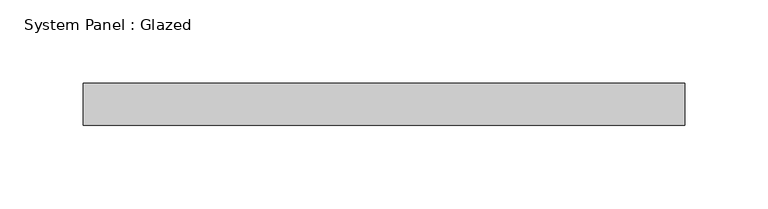
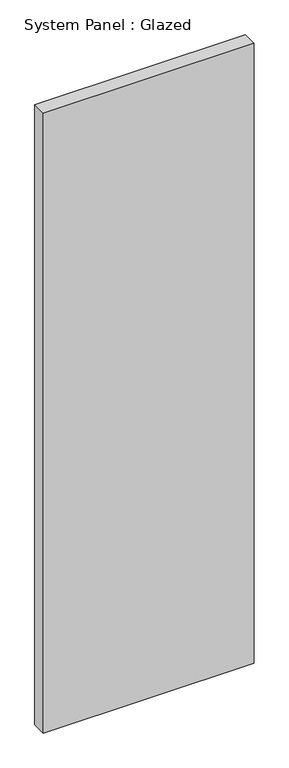
"""IFC4 building model written with IfcOpenShell, lengths in millimetres: plate geometry, System Panel : Glazed."""

from ifc_helpers import new_model, si_unit, origin, origin_with_axes, place, context, project, spatial, polyline, outline, extrude, source, transform, mapped, element, save


def system_panel_glazed_db5a8f8c(model_context):
    return source(origin(), model_context, "Body", "SweptSolid", [
        extrude(outline(polyline([(180.975, 19.05), (-180.975, 19.05), (-180.975, 44.45), (180.975, 44.45), (180.975, 19.05)])), origin_with_axes(), (0.0, 0.0, 1.0), 1123.95),
    ])


if __name__ == "__main__":
    model = new_model("IFC4")
    model_context = context("Model", 3, world=origin())
    ifc_project = project(units=[si_unit("LENGTHUNIT", "METRE", prefix="MILLI")], contexts=[model_context])
    site = spatial("IfcSite", under=ifc_project)
    building = spatial("IfcBuilding", under=site)
    placement = place(None, origin())
    system_panel_glazed_shape = system_panel_glazed_db5a8f8c(model_context)
    element("IfcPlate", 1, ObjectType="System Panel : Glazed", at=placement, inside=building, context=model_context, shape_type="MappedRepresentation", body=[
        mapped(system_panel_glazed_shape, transform((0.0, 0.0, 0.0), x_axis=(1.0, 0.0, 0.0), y_axis=(0.0, 1.0, 0.0), z_axis=(0.0, 0.0, 1.0))),
    ])
    save(model, "model.ifc")

# Revit data of these elements
# Type "System Panel : Glazed"
#   Construction Type Id = "GSP4R"
#   Analytic Construction = "1/8 in Pilkington single glazing"
#   Visual Light Transmittance = 0.9
#   Solar Heat Gain Coefficient = 0.86
#   Heat Transfer Coefficient (U) = 1.18115 BTU/(h·ft²·°F)
#   Define Thermal Properties by = 1
# Element 1 (IfcPlate, "System Panel : Glazed")
#   Materials on its faces: "Glass"
# Materials
#   "Glass": class "Glass", colour RGB 0 128 192, transparency 0.75, Description = "Soda Lime Glass", Cost = 0
